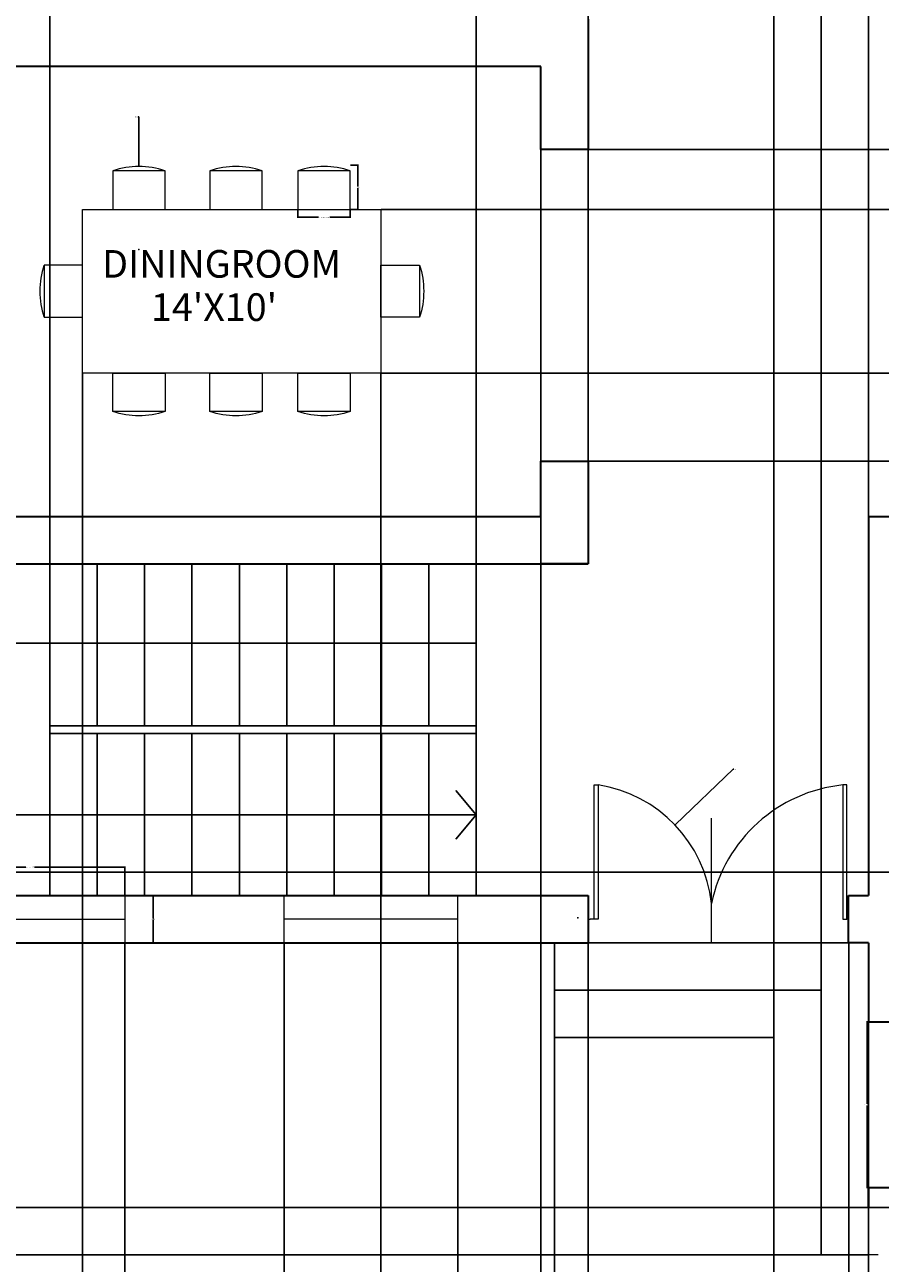
# Model space of a CAD drawing. Units: inches. Extents: x 2863 to 3499, y 1212 to 2136.
# Tile 3 of 7: x 2991 to 3208, y 1372 to 1686. Entities that reach past the tile are written whole.
import ezdxf

# ---------------------------------------------------------------- set-up
doc = ezdxf.new("R2010")
doc.units = ezdxf.units.IN
doc.linetypes.add('DASHED2', pattern=[9.525, 6.35, -3.175])
for name, color, linetype, lineweight in [('A-ANNO-DIMS', 2, 'Continuous', 18), ('A-AREA-IDEN', 7, 'Continuous', 18), ('A-DOOR', 221, 'Continuous', 18), ('A-FLOR-OVHD', 51, 'DASHED2', 18), ('A-FLOR-STRS', 51, 'Continuous', 25), ('A-FURN', 131, 'Continuous', 18), ('A-GLAZ', 191, 'Continuous', 18), ('A-WALL', 51, 'Continuous', 35)]:
    doc.layers.add(name, color=color, linetype=linetype, lineweight=lineweight)
doc.styles.get("Standard").update_dxf_attribs({"font": 'arial.ttf'})
doc.dimstyles.get("Standard").update_dxf_attribs({"dimtxt": 0.18, "dimasz": 0.18, "dimexe": 0.18, "dimexo": 0.0625, "dimgap": 0.09, "dimtad": 0, "dimtih": 1, "dimtoh": 1, "dimdec": 4, "dimzin": 0, "dimdsep": 46, "dimtxsty": 'Standard', "dimcen": 0.09, "dimadec": 0, "dimazin": 0, "dimtfac": 1, "dimtdec": 4, "dimtofl": 0, "dimtmove": 0, "dimatfit": 3, "dimfxl": 1, "dimtolj": 1, "dimtzin": 0, "dimarcsym": 0})

# ---------------------------------------------------------------- blocks, each defined once
blk = doc.blocks.new('CHAIR-DINING')
blk.add_lwpolyline([(0, 0), (13.22, 0), (13.22, 9.77), (0, 9.77)], close=True)
blk.add_arc((6.61, -10.16), 21, 71.6601, 108.3399)
blk = doc.blocks.new('WINDOW-44IN')
for p, q in [((12, 44), (0, 44)), ((6, 44), (6, 0)), ((12, 0), (0, 0))]:
    blk.add_line(p, q)
blk = doc.blocks.new('WINDOW-48IN')
for p, q in [((12, 48), (0, 48)), ((6, 48), (6, 0)), ((12, 0), (0, 0))]:
    blk.add_line(p, q)
blk = doc.blocks.new('*D17')
at = {"layer": 'A-ANNO-DIMS', "color": 0, "lineweight": -2, "transparency": 16777216}
for p, q in [((3060.4, 1638.9), (3060.4, 1636.8)), ((3073.61, 1638.9), (3073.61, 1636.8)), ((3060.58, 1636.98), (3065.58, 1636.98)), ((3073.43, 1636.98), (3068.43, 1636.98))]:
    blk.add_line(p, q, dxfattribs=at)
at = {"layer": 'A-ANNO-DIMS', "color": 0, "transparency": 16777216}
for points in [[(3060.58, 1637.01), (3060.58, 1636.95), (3060.4, 1636.98)], [(3073.43, 1637.01), (3073.43, 1636.95), (3073.61, 1636.98)]]:
    blk.add_solid(points, dxfattribs=at)
at = {"layer": 'Defpoints', "color": 0, "transparency": 16777216}
for p in [(3060.4, 1638.96), (3073.61, 1638.96), (3073.61, 1636.98)]:
    blk.add_point(p, dxfattribs=at)
at = {"layer": 'A-ANNO-DIMS', "color": 0, "transparency": 16777216, "insert": (3067, 1636.98), "char_height": 0.18, "attachment_point": 5}
blk.add_mtext('\\A1;DINING CHAIR 13 TYP.', dxfattribs=at)
blk = doc.blocks.new('*D18')
at = {"layer": 'A-ANNO-DIMS', "color": 0, "lineweight": -2, "transparency": 16777216}
for p, q in [((3073.67, 1650.15), (3075.77, 1650.15)), ((3075.59, 1649.97), (3075.59, 1644.74)), ((3075.59, 1639.14), (3075.59, 1644.37)), ((3073.67, 1638.96), (3075.77, 1638.96))]:
    blk.add_line(p, q, dxfattribs=at)
at = {"layer": 'A-ANNO-DIMS', "color": 0, "transparency": 16777216}
for points in [[(3075.56, 1649.97), (3075.62, 1649.97), (3075.59, 1650.15)], [(3075.56, 1639.14), (3075.62, 1639.14), (3075.59, 1638.96)]]:
    blk.add_solid(points, dxfattribs=at)
at = {"layer": 'Defpoints', "color": 0, "transparency": 16777216}
for p in [(3073.61, 1650.15), (3075.59, 1650.15), (3073.61, 1638.96)]:
    blk.add_point(p, dxfattribs=at)
at = {"layer": 'A-ANNO-DIMS', "color": 0, "transparency": 16777216, "insert": (3075.59, 1644.56), "char_height": 0.18, "attachment_point": 5}
blk.add_mtext('\\A1;11 TYP.', dxfattribs=at)
blk = doc.blocks.new('*D33')
at = {"layer": 'A-ANNO-DIMS', "color": 0, "lineweight": -2, "transparency": 16777216}
for p, q in [((2968.53, 1465.23), (2968.53, 1472.55)), ((2968.71, 1472.37), (2991.41, 1472.37)), ((3016.35, 1472.37), (2993.64, 1472.37)), ((3016.53, 1465.23), (3016.53, 1472.55))]:
    blk.add_line(p, q, dxfattribs=at)
at = {"layer": 'A-ANNO-DIMS', "color": 0, "transparency": 16777216}
for points in [[(2968.71, 1472.4), (2968.71, 1472.34), (2968.53, 1472.37)], [(3016.35, 1472.4), (3016.35, 1472.34), (3016.53, 1472.37)]]:
    blk.add_solid(points, dxfattribs=at)
at = {"layer": 'Defpoints', "color": 0, "transparency": 16777216}
for p in [(2968.53, 1472.37), (2968.53, 1465.17), (3016.53, 1465.17)]:
    blk.add_point(p, dxfattribs=at)
at = {"layer": 'A-ANNO-DIMS', "color": 0, "transparency": 16777216, "insert": (2992.53, 1472.37), "char_height": 0.18, "attachment_point": 5}
blk.add_mtext('\\A1;WINDOW 48 TYP.', dxfattribs=at)
blk = doc.blocks.new('*D34')
at = {"layer": 'A-ANNO-DIMS', "color": 0, "lineweight": -2, "transparency": 16777216}
for p, q in [((3016.59, 1465.17), (3023.91, 1465.17)), ((3023.73, 1464.99), (3023.73, 1459.35)), ((3023.73, 1453.35), (3023.73, 1458.98)), ((3016.59, 1453.17), (3023.91, 1453.17))]:
    blk.add_line(p, q, dxfattribs=at)
at = {"layer": 'A-ANNO-DIMS', "color": 0, "transparency": 16777216}
for points in [[(3023.7, 1464.99), (3023.76, 1464.99), (3023.73, 1465.17)], [(3023.7, 1453.35), (3023.76, 1453.35), (3023.73, 1453.17)]]:
    blk.add_solid(points, dxfattribs=at)
at = {"layer": 'Defpoints', "color": 0, "transparency": 16777216}
for p in [(3016.53, 1465.17), (3023.73, 1465.17), (3016.53, 1453.17)]:
    blk.add_point(p, dxfattribs=at)
at = {"layer": 'A-ANNO-DIMS', "color": 0, "transparency": 16777216, "insert": (3023.73, 1459.17), "char_height": 0.18, "attachment_point": 5}
blk.add_mtext('\\A1;12 TYP.', dxfattribs=at)
blk = doc.blocks.new('*D39')
at = {"layer": 'A-ANNO-DIMS', "color": 0, "lineweight": -2, "transparency": 16777216}
for p, q in [((3210.85, 1433.18), (3204.43, 1433.18)), ((3204.61, 1433), (3204.61, 1412.36)), ((3204.61, 1391.35), (3204.61, 1411.99)), ((3210.85, 1391.17), (3204.43, 1391.17))]:
    blk.add_line(p, q, dxfattribs=at)
at = {"layer": 'A-ANNO-DIMS', "color": 0, "transparency": 16777216}
for points in [[(3204.58, 1433), (3204.64, 1433), (3204.61, 1433.18)], [(3204.58, 1391.35), (3204.64, 1391.35), (3204.61, 1391.17)]]:
    blk.add_solid(points, dxfattribs=at)
at = {"layer": 'Defpoints', "color": 0, "transparency": 16777216}
for p in [(3204.61, 1433.18), (3210.92, 1433.18), (3210.92, 1391.17)]:
    blk.add_point(p, dxfattribs=at)
at = {"layer": 'A-ANNO-DIMS', "color": 0, "transparency": 16777216, "insert": (3204.61, 1412.17), "char_height": 0.18, "attachment_point": 5}
blk.add_mtext('\\A1;DOOR 42 TYP.', dxfattribs=at)
blk = doc.blocks.new('*D69')
at = {"layer": 'A-ANNO-DIMS', "color": 0, "lineweight": -2, "transparency": 16777216}
for p, q in [((3204.85, 1453.17), (2862.72, 1453.17)), ((2862.9, 1452.99), (2862.9, 1413.85)), ((2862.9, 1374.35), (2862.9, 1413.48)), ((3204.85, 1374.17), (2862.72, 1374.17))]:
    blk.add_line(p, q, dxfattribs=at)
at = {"layer": 'A-ANNO-DIMS', "color": 0, "transparency": 16777216}
for points in [[(2862.87, 1452.99), (2862.93, 1452.99), (2862.9, 1453.17)], [(2862.87, 1374.35), (2862.93, 1374.35), (2862.9, 1374.17)]]:
    blk.add_solid(points, dxfattribs=at)
at = {"layer": 'Defpoints', "color": 0, "transparency": 16777216}
for p in [(3204.92, 1453.17), (2862.9, 1374.17), (3204.92, 1374.17)]:
    blk.add_point(p, dxfattribs=at)
at = {"layer": 'A-ANNO-DIMS', "color": 0, "transparency": 16777216, "insert": (2862.9, 1413.67), "char_height": 0.18, "attachment_point": 5}
blk.add_mtext('\\A1;79', dxfattribs=at)
blk = doc.blocks.new('*D70')
at = {"layer": 'A-ANNO-DIMS', "color": 0, "lineweight": -2, "transparency": 16777216}
for p, q in [((2940.92, 1453.1), (2940.92, 1211.97)), ((3204.92, 1374.1), (3204.92, 1211.97)), ((2941.1, 1212.15), (3072.63, 1212.15)), ((3204.74, 1212.15), (3073.21, 1212.15))]:
    blk.add_line(p, q, dxfattribs=at)
at = {"layer": 'A-ANNO-DIMS', "color": 0, "transparency": 16777216}
for points in [[(2941.1, 1212.18), (2941.1, 1212.12), (2940.92, 1212.15)], [(3204.74, 1212.18), (3204.74, 1212.12), (3204.92, 1212.15)]]:
    blk.add_solid(points, dxfattribs=at)
at = {"layer": 'Defpoints', "color": 0, "transparency": 16777216}
for p in [(2940.92, 1453.17), (3204.92, 1374.17), (3204.92, 1212.15)]:
    blk.add_point(p, dxfattribs=at)
at = {"layer": 'A-ANNO-DIMS', "color": 0, "transparency": 16777216, "insert": (3072.92, 1212.15), "char_height": 0.18, "attachment_point": 5}
blk.add_mtext('\\A1;264', dxfattribs=at)
blk = doc.blocks.new('*D71')
at = {"layer": 'A-ANNO-DIMS', "color": 0, "lineweight": -2, "transparency": 16777216}
for p, q in [((3204.92, 1374.1), (3204.92, 1211.97)), ((3420.92, 1374.1), (3420.92, 1211.97)), ((3205.1, 1212.15), (3312.63, 1212.15)), ((3420.74, 1212.15), (3313.21, 1212.15))]:
    blk.add_line(p, q, dxfattribs=at)
at = {"layer": 'A-ANNO-DIMS', "color": 0, "transparency": 16777216}
for points in [[(3205.1, 1212.18), (3205.1, 1212.12), (3204.92, 1212.15)], [(3420.74, 1212.18), (3420.74, 1212.12), (3420.92, 1212.15)]]:
    blk.add_solid(points, dxfattribs=at)
at = {"layer": 'Defpoints', "color": 0, "transparency": 16777216}
for p in [(3204.92, 1374.17), (3420.92, 1374.17), (3420.92, 1212.15)]:
    blk.add_point(p, dxfattribs=at)
at = {"layer": 'A-ANNO-DIMS', "color": 0, "transparency": 16777216, "insert": (3312.92, 1212.15), "char_height": 0.18, "attachment_point": 5}
blk.add_mtext('\\A1;216', dxfattribs=at)
blk = doc.blocks.new('*D72')
at = {"layer": 'A-ANNO-DIMS', "color": 0, "lineweight": -2, "transparency": 16777216}
for p, q in [((3133.92, 1549.23), (3133.92, 2136.37)), ((3204.92, 1561.23), (3204.92, 2136.37)), ((3134.1, 2136.19), (3169.22, 2136.19)), ((3204.74, 2136.19), (3169.62, 2136.19))]:
    blk.add_line(p, q, dxfattribs=at)
at = {"layer": 'A-ANNO-DIMS', "color": 0, "transparency": 16777216}
for points in [[(3134.1, 2136.22), (3134.1, 2136.16), (3133.92, 2136.19)], [(3204.74, 2136.22), (3204.74, 2136.16), (3204.92, 2136.19)]]:
    blk.add_solid(points, dxfattribs=at)
at = {"layer": 'Defpoints', "color": 0, "transparency": 16777216}
for p in [(3204.92, 2136.19), (3204.92, 1561.17), (3133.92, 1549.17)]:
    blk.add_point(p, dxfattribs=at)
at = {"layer": 'A-ANNO-DIMS', "color": 0, "transparency": 16777216, "insert": (3169.42, 2136.19), "char_height": 0.18, "attachment_point": 5}
blk.add_mtext('\\A1;71', dxfattribs=at)
blk = doc.blocks.new('*D74')
at = {"layer": 'A-ANNO-DIMS', "color": 0, "lineweight": -2, "transparency": 16777216}
for p, q in [((3408.85, 1471.09), (2862.72, 1471.09)), ((2862.9, 1470.91), (2862.9, 1428.81)), ((2862.9, 1386.35), (2862.9, 1428.44)), ((3408.85, 1386.17), (2862.72, 1386.17))]:
    blk.add_line(p, q, dxfattribs=at)
at = {"layer": 'A-ANNO-DIMS', "color": 0, "transparency": 16777216}
for points in [[(2862.87, 1470.91), (2862.93, 1470.91), (2862.9, 1471.09)], [(2862.87, 1386.35), (2862.93, 1386.35), (2862.9, 1386.17)]]:
    blk.add_solid(points, dxfattribs=at)
at = {"layer": 'Defpoints', "color": 0, "transparency": 16777216}
for p in [(3408.92, 1471.09), (2862.9, 1386.17), (3408.92, 1386.17)]:
    blk.add_point(p, dxfattribs=at)
at = {"layer": 'A-ANNO-DIMS', "color": 0, "transparency": 16777216, "insert": (2862.9, 1428.63), "char_height": 0.18, "attachment_point": 5}
blk.add_mtext('\\A1;84.92', dxfattribs=at)
blk = doc.blocks.new('*D76')
at = {"layer": 'A-ANNO-DIMS', "color": 0, "lineweight": -2, "transparency": 16777216}
for p, q in [((2952.92, 1675.1), (2952.92, 1211.97)), ((3121.92, 1675.1), (3121.92, 1211.97)), ((2953.1, 1212.15), (3037.14, 1212.15)), ((3121.74, 1212.15), (3037.7, 1212.15))]:
    blk.add_line(p, q, dxfattribs=at)
at = {"layer": 'A-ANNO-DIMS', "color": 0, "transparency": 16777216}
for points in [[(2953.1, 1212.18), (2953.1, 1212.12), (2952.92, 1212.15)], [(3121.74, 1212.18), (3121.74, 1212.12), (3121.92, 1212.15)]]:
    blk.add_solid(points, dxfattribs=at)
at = {"layer": 'Defpoints', "color": 0, "transparency": 16777216}
for p in [(2952.92, 1675.17), (3121.92, 1675.17), (3121.92, 1212.15)]:
    blk.add_point(p, dxfattribs=at)
at = {"layer": 'A-ANNO-DIMS', "color": 0, "transparency": 16777216, "insert": (3037.42, 1212.15), "char_height": 0.18, "attachment_point": 5}
blk.add_mtext('\\A1;169', dxfattribs=at)
blk = doc.blocks.new('*D77')
at = {"layer": 'A-ANNO-DIMS', "color": 0, "lineweight": -2, "transparency": 16777216}
for p, q in [((2997.55, 1549.23), (2997.55, 2136.37)), ((3105.55, 1549.23), (3105.55, 2136.37)), ((2997.73, 2136.19), (3051.27, 2136.19)), ((3105.37, 2136.19), (3051.83, 2136.19))]:
    blk.add_line(p, q, dxfattribs=at)
at = {"layer": 'A-ANNO-DIMS', "color": 0, "transparency": 16777216}
for points in [[(2997.73, 2136.22), (2997.73, 2136.16), (2997.55, 2136.19)], [(3105.37, 2136.22), (3105.37, 2136.16), (3105.55, 2136.19)]]:
    blk.add_solid(points, dxfattribs=at)
at = {"layer": 'Defpoints', "color": 0, "transparency": 16777216}
for p in [(3105.55, 2136.19), (2997.55, 1549.17), (3105.55, 1549.17)]:
    blk.add_point(p, dxfattribs=at)
at = {"layer": 'A-ANNO-DIMS', "color": 0, "transparency": 16777216, "insert": (3051.55, 2136.19), "char_height": 0.18, "attachment_point": 5}
blk.add_mtext('\\A1;108', dxfattribs=at)
blk = doc.blocks.new('*D79')
at = {"layer": 'A-ANNO-DIMS', "color": 0, "lineweight": -2, "transparency": 16777216}
for p, q in [((3005.82, 1597.44), (3005.82, 1211.97)), ((3081.41, 1597.44), (3081.41, 1211.97)), ((3006, 1212.15), (3043.23, 1212.15)), ((3081.23, 1212.15), (3044.01, 1212.15))]:
    blk.add_line(p, q, dxfattribs=at)
at = {"layer": 'A-ANNO-DIMS', "color": 0, "transparency": 16777216}
for points in [[(3006, 1212.18), (3006, 1212.12), (3005.82, 1212.15)], [(3081.23, 1212.18), (3081.23, 1212.12), (3081.41, 1212.15)]]:
    blk.add_solid(points, dxfattribs=at)
at = {"layer": 'Defpoints', "color": 0, "transparency": 16777216}
for p in [(3005.82, 1597.5), (3081.41, 1597.5), (3081.41, 1212.15)]:
    blk.add_point(p, dxfattribs=at)
at = {"layer": 'A-ANNO-DIMS', "color": 0, "transparency": 16777216, "insert": (3043.62, 1212.15), "char_height": 0.18, "attachment_point": 5}
blk.add_mtext('\\A1;75.59', dxfattribs=at)
blk = doc.blocks.new('*D80')
at = {"layer": 'A-ANNO-DIMS', "color": 0, "lineweight": -2, "transparency": 16777216}
for p, q in [((3081.48, 1638.96), (3499.12, 1638.96)), ((3498.94, 1638.78), (3498.94, 1618.41)), ((3498.94, 1597.68), (3498.94, 1618.05)), ((3081.48, 1597.5), (3499.12, 1597.5))]:
    blk.add_line(p, q, dxfattribs=at)
at = {"layer": 'A-ANNO-DIMS', "color": 0, "transparency": 16777216}
for points in [[(3498.91, 1638.78), (3498.97, 1638.78), (3498.94, 1638.96)], [(3498.91, 1597.68), (3498.97, 1597.68), (3498.94, 1597.5)]]:
    blk.add_solid(points, dxfattribs=at)
at = {"layer": 'Defpoints', "color": 0, "transparency": 16777216}
for p in [(3081.41, 1638.96), (3498.94, 1638.96), (3081.41, 1597.5)]:
    blk.add_point(p, dxfattribs=at)
at = {"layer": 'A-ANNO-DIMS', "color": 0, "transparency": 16777216, "insert": (3498.94, 1618.23), "char_height": 0.18, "attachment_point": 5}
blk.add_mtext('\\A1;41.46', dxfattribs=at)
blk = doc.blocks.new('*D81')
at = {"layer": 'A-ANNO-DIMS', "color": 0, "lineweight": -2, "transparency": 16777216}
for p, q in [((3133.92, 1453.1), (3133.92, 1211.97)), ((3199.92, 1453.1), (3199.92, 1211.97)), ((3134.1, 1212.15), (3166.7, 1212.15)), ((3199.74, 1212.15), (3167.14, 1212.15))]:
    blk.add_line(p, q, dxfattribs=at)
at = {"layer": 'A-ANNO-DIMS', "color": 0, "transparency": 16777216}
for points in [[(3134.1, 1212.18), (3134.1, 1212.12), (3133.92, 1212.15)], [(3199.74, 1212.18), (3199.74, 1212.12), (3199.92, 1212.15)]]:
    blk.add_solid(points, dxfattribs=at)
at = {"layer": 'Defpoints', "color": 0, "transparency": 16777216}
for p in [(3133.92, 1453.17), (3199.92, 1453.17), (3199.92, 1212.15)]:
    blk.add_point(p, dxfattribs=at)
at = {"layer": 'A-ANNO-DIMS', "color": 0, "transparency": 16777216, "insert": (3166.92, 1212.15), "char_height": 0.18, "attachment_point": 5}
blk.add_mtext('\\A1;66', dxfattribs=at)
blk = doc.blocks.new('*D82')
at = {"layer": 'A-ANNO-DIMS', "color": 0, "lineweight": -2, "transparency": 16777216}
for p, q in [((3121.98, 1654.17), (3499.12, 1654.17)), ((3498.94, 1653.99), (3498.94, 1614.85)), ((3498.94, 1575.35), (3498.94, 1614.48)), ((3121.98, 1575.17), (3499.12, 1575.17))]:
    blk.add_line(p, q, dxfattribs=at)
at = {"layer": 'A-ANNO-DIMS', "color": 0, "transparency": 16777216}
for points in [[(3498.91, 1653.99), (3498.97, 1653.99), (3498.94, 1654.17)], [(3498.91, 1575.35), (3498.97, 1575.35), (3498.94, 1575.17)]]:
    blk.add_solid(points, dxfattribs=at)
at = {"layer": 'Defpoints', "color": 0, "transparency": 16777216}
for p in [(3121.92, 1654.17), (3498.94, 1654.17), (3121.92, 1575.17)]:
    blk.add_point(p, dxfattribs=at)
at = {"layer": 'A-ANNO-DIMS', "color": 0, "transparency": 16777216, "insert": (3498.94, 1614.67), "char_height": 0.18, "attachment_point": 5}
blk.add_mtext('\\A1;79', dxfattribs=at)
blk = doc.blocks.new('*D102')
at = {"layer": 'A-ANNO-DIMS', "color": 0, "lineweight": -2, "transparency": 16777216}
for p, q in [((3016.53, 1453.1), (3016.53, 1211.97)), ((3056.9, 1453.1), (3056.9, 1211.97)), ((3016.71, 1212.15), (3036.31, 1212.15)), ((3056.72, 1212.15), (3037.11, 1212.15))]:
    blk.add_line(p, q, dxfattribs=at)
at = {"layer": 'A-ANNO-DIMS', "color": 0, "transparency": 16777216}
for points in [[(3016.71, 1212.18), (3016.71, 1212.12), (3016.53, 1212.15)], [(3056.72, 1212.18), (3056.72, 1212.12), (3056.9, 1212.15)]]:
    blk.add_solid(points, dxfattribs=at)
at = {"layer": 'Defpoints', "color": 0, "transparency": 16777216}
for p in [(3016.53, 1453.17), (3056.9, 1453.17), (3056.9, 1212.15)]:
    blk.add_point(p, dxfattribs=at)
at = {"layer": 'A-ANNO-DIMS', "color": 0, "transparency": 16777216, "insert": (3036.71, 1212.15), "char_height": 0.18, "attachment_point": 5}
blk.add_mtext('\\A1;40.37', dxfattribs=at)
blk = doc.blocks.new('*D103')
at = {"layer": 'A-ANNO-DIMS', "color": 0, "lineweight": -2, "transparency": 16777216}
for p, q in [((3100.9, 1453.1), (3100.9, 1211.97)), ((3133.92, 1453.1), (3133.92, 1211.97)), ((3101.08, 1212.15), (3117.01, 1212.15)), ((3133.74, 1212.15), (3117.8, 1212.15))]:
    blk.add_line(p, q, dxfattribs=at)
at = {"layer": 'A-ANNO-DIMS', "color": 0, "transparency": 16777216}
for points in [[(3101.08, 1212.18), (3101.08, 1212.12), (3100.9, 1212.15)], [(3133.74, 1212.18), (3133.74, 1212.12), (3133.92, 1212.15)]]:
    blk.add_solid(points, dxfattribs=at)
at = {"layer": 'Defpoints', "color": 0, "transparency": 16777216}
for p in [(3100.9, 1453.17), (3133.92, 1453.17), (3133.92, 1212.15)]:
    blk.add_point(p, dxfattribs=at)
at = {"layer": 'A-ANNO-DIMS', "color": 0, "transparency": 16777216, "insert": (3117.41, 1212.15), "char_height": 0.18, "attachment_point": 5}
blk.add_mtext('\\A1;33.02', dxfattribs=at)
blk = doc.blocks.new('*D109')
at = {"layer": 'A-ANNO-DIMS', "color": 0, "lineweight": -2, "transparency": 16777216}
for p, q in [((3125.36, 1429.1), (3125.36, 1211.97)), ((3180.92, 1429.1), (3180.92, 1211.97)), ((3125.54, 1212.15), (3152.74, 1212.15)), ((3180.74, 1212.15), (3153.53, 1212.15))]:
    blk.add_line(p, q, dxfattribs=at)
at = {"layer": 'A-ANNO-DIMS', "color": 0, "transparency": 16777216}
for points in [[(3125.54, 1212.18), (3125.54, 1212.12), (3125.36, 1212.15)], [(3180.74, 1212.18), (3180.74, 1212.12), (3180.92, 1212.15)]]:
    blk.add_solid(points, dxfattribs=at)
at = {"layer": 'Defpoints', "color": 0, "transparency": 16777216}
for p in [(3125.36, 1429.17), (3180.92, 1429.17), (3180.92, 1212.15)]:
    blk.add_point(p, dxfattribs=at)
at = {"layer": 'A-ANNO-DIMS', "color": 0, "transparency": 16777216, "insert": (3153.14, 1212.15), "char_height": 0.18, "attachment_point": 5}
blk.add_mtext('\\A1;55.56', dxfattribs=at)
blk = doc.blocks.new('*D110')
at = {"layer": 'A-ANNO-DIMS', "color": 0, "lineweight": -2, "transparency": 16777216}
for p, q in [((3180.92, 1374.23), (3180.92, 2136.37)), ((3192.92, 1374.23), (3192.92, 2136.37)), ((3181.1, 2136.19), (3186.71, 2136.19)), ((3192.74, 2136.19), (3187.13, 2136.19))]:
    blk.add_line(p, q, dxfattribs=at)
at = {"layer": 'A-ANNO-DIMS', "color": 0, "transparency": 16777216}
for points in [[(3181.1, 2136.22), (3181.1, 2136.16), (3180.92, 2136.19)], [(3192.74, 2136.22), (3192.74, 2136.16), (3192.92, 2136.19)]]:
    blk.add_solid(points, dxfattribs=at)
at = {"layer": 'Defpoints', "color": 0, "transparency": 16777216}
for p in [(3192.92, 2136.19), (3180.92, 1374.17), (3192.92, 1374.17)]:
    blk.add_point(p, dxfattribs=at)
at = {"layer": 'A-ANNO-DIMS', "color": 0, "transparency": 16777216, "insert": (3186.92, 2136.19), "char_height": 0.18, "attachment_point": 5}
blk.add_mtext('\\A1;12', dxfattribs=at)
blk = doc.blocks.new('*D111')
at = {"layer": 'A-ANNO-DIMS', "color": 0, "lineweight": -2, "transparency": 16777216}
for p, q in [((2952.92, 1549.23), (2952.92, 2136.37)), ((2997.55, 1549.23), (2997.55, 2136.37)), ((2953.1, 2136.19), (2974.83, 2136.19)), ((2997.37, 2136.19), (2975.63, 2136.19))]:
    blk.add_line(p, q, dxfattribs=at)
at = {"layer": 'A-ANNO-DIMS', "color": 0, "transparency": 16777216}
for points in [[(2953.1, 2136.22), (2953.1, 2136.16), (2952.92, 2136.19)], [(2997.37, 2136.22), (2997.37, 2136.16), (2997.55, 2136.19)]]:
    blk.add_solid(points, dxfattribs=at)
at = {"layer": 'Defpoints', "color": 0, "transparency": 16777216}
for p in [(2997.55, 2136.19), (2952.92, 1549.17), (2997.55, 1549.17)]:
    blk.add_point(p, dxfattribs=at)
at = {"layer": 'A-ANNO-DIMS', "color": 0, "transparency": 16777216, "insert": (2975.23, 2136.19), "char_height": 0.18, "attachment_point": 5}
blk.add_mtext('\\A1;44.63', dxfattribs=at)
blk = doc.blocks.new('*D115')
at = {"layer": 'A-ANNO-DIMS', "color": 0, "lineweight": -2, "transparency": 16777216}
for p, q in [((3170.64, 1497.15), (3156.03, 1483.17)), ((3170.82, 1497.15), (3170.64, 1497.15)), ((3131.24, 1459.55), (3131.42, 1459.55)), ((3131.33, 1459.46), (3131.33, 1459.64))]:
    blk.add_line(p, q, dxfattribs=at)
at = {"layer": 'A-ANNO-DIMS', "color": 0, "transparency": 16777216}
blk.add_solid([(3156.01, 1483.2), (3156.05, 1483.15), (3155.9, 1483.05)], dxfattribs=at)
at = {"layer": 'Defpoints', "color": 0, "transparency": 16777216}
for p in [(3155.9, 1483.05), (3131.33, 1459.55)]:
    blk.add_point(p, dxfattribs=at)
at = {"layer": 'A-ANNO-DIMS', "color": 0, "transparency": 16777216, "insert": (3171.12, 1497.15), "char_height": 0.18, "attachment_point": 5}
blk.add_mtext('\\A1;R34', dxfattribs=at)
blk = doc.blocks.new('*D119')
at = {"layer": 'A-ANNO-DIMS', "color": 0, "lineweight": -2, "transparency": 16777216}
for p, q in [((3019.91, 1662.4), (3020.09, 1662.4)), ((3020.09, 1662.4), (3020.09, 1649.98)), ((3020.01, 1628.8), (3020.19, 1628.8)), ((3020.1, 1628.71), (3020.1, 1628.89))]:
    blk.add_line(p, q, dxfattribs=at)
at = {"layer": 'A-ANNO-DIMS', "color": 0, "transparency": 16777216}
blk.add_solid([(3020.12, 1649.98), (3020.06, 1649.98), (3020.09, 1649.8)], dxfattribs=at)
at = {"layer": 'Defpoints', "color": 0, "transparency": 16777216}
for p in [(3020.09, 1649.8), (3020.1, 1628.8)]:
    blk.add_point(p, dxfattribs=at)
at = {"layer": 'A-ANNO-DIMS', "color": 0, "transparency": 16777216, "insert": (3019.43, 1662.4), "char_height": 0.18, "attachment_point": 5}
blk.add_mtext('\\A1;4X R21', dxfattribs=at)

msp = doc.modelspace()

# ---------------------------------------------------------------- linework, layer by layer
at = {"layer": 'A-DOOR'}
for p, q in [((3135.4168, 1459.1651), (3135.4168, 1493.1651)), ((3135.4168, 1493.1651), (3136.4168, 1493.1651)), ((3136.4168, 1493.1651), (3136.4168, 1459.1651)), ((3199.4168, 1493.1651), (3198.4168, 1493.1651)), ((3198.4168, 1493.1651), (3198.4168, 1459.1651)), ((3199.4168, 1459.1651), (3199.4168, 1493.1651)), ((3165.1366, 1453.1651), (3165.1366, 1484.7256)), ((3133.9168, 1459.1651), (3134.4168, 1459.1651)), ((3135.4168, 1459.1651), (3134.4168, 1459.1651)), ((3136.4168, 1459.1651), (3135.4168, 1459.1651)), ((3198.4168, 1459.1651), (3199.4168, 1459.1651)), ((3199.9168, 1459.1651), (3199.4168, 1459.1651))]:
    msp.add_line(p, q, dxfattribs=at)
for centre, radius, start, end in [((3131.3266, 1459.5483), 34, 6.059429, 81.389827), ((3202.3338, 1455.3675), 38, 95.916573, 168.201616)]:
    msp.add_arc(centre, radius, start, end, dxfattribs=at)
at = {"layer": 'A-FLOR-OVHD'}
for p, q in [((3121.9168, 1654.1651), (3121.9168, 1575.1651)), ((3133.9168, 1654.1651), (3133.9168, 1575.1651)), ((2952.9168, 1386.1651), (3204.9168, 1386.1651)), ((3216.9168, 1374.1651), (2940.9168, 1374.1651))]:
    msp.add_line(p, q, dxfattribs=at)
at = {"layer": 'A-FLOR-STRS'}
for p, q in [((2997.5458, 1549.1651), (2997.5458, 1465.1651)), ((3009.5458, 1549.1651), (3009.5458, 1508.1651)), ((3021.5458, 1549.1651), (3021.5458, 1508.1651)), ((3033.5458, 1549.1651), (3033.5458, 1508.1651)), ((3045.5458, 1549.1651), (3045.5458, 1508.1651)), ((3057.5458, 1549.1651), (3057.5458, 1508.1651)), ((3069.5458, 1549.1651), (3069.5458, 1508.1651)), ((3081.5458, 1549.1651), (3081.5458, 1508.1651)), ((3093.5458, 1549.1651), (3093.5458, 1508.1651)), ((3105.5458, 1549.1651), (3105.5458, 1465.1651)), ((3105.5458, 1529.0656), (2976.4727, 1529.0656)), ((3105.5458, 1508.1651), (2997.5458, 1508.1651)), ((3105.5458, 1506.1651), (2997.5458, 1506.1651)), ((3009.5458, 1506.1651), (3009.5458, 1465.1651)), ((3021.5458, 1506.1651), (3021.5458, 1465.1651)), ((3033.5458, 1506.1651), (3033.5458, 1465.1651)), ((3045.5458, 1506.1651), (3045.5458, 1465.1651)), ((3057.5458, 1506.1651), (3057.5458, 1465.1651)), ((3069.5458, 1506.1651), (3069.5458, 1465.1651)), ((3081.5458, 1506.1651), (3081.5458, 1465.1651)), ((3093.5458, 1506.1651), (3093.5458, 1465.1651)), ((3105.5458, 1485.602), (3100.4035, 1491.7303)), ((2976.4727, 1485.602), (3105.5458, 1485.602)), ((3105.5458, 1485.602), (3100.4035, 1479.4736)), ((3125.3565, 1453.1651), (3204.9168, 1453.1651)), ((3125.3565, 1441.1651), (3125.3565, 1453.1651)), ((3204.9168, 1453.1651), (3204.9168, 1374.1651)), ((3192.9168, 1441.1651), (3125.3565, 1441.1651)), ((3125.3565, 1429.1651), (3125.3565, 1441.1651)), ((3192.9168, 1374.1651), (3192.9168, 1441.1651)), ((3180.9168, 1429.1651), (3125.3565, 1429.1651)), ((3180.9168, 1374.1651), (3180.9168, 1429.1651)), ((3192.9168, 1374.1651), (3180.9168, 1374.1651)), ((3204.9168, 1374.1651), (3192.9168, 1374.1651))]:
    msp.add_line(p, q, dxfattribs=at)
at = {"layer": 'A-FURN'}
msp.add_lwpolyline([(3005.8227, 1638.9588), (3081.415, 1638.9588), (3081.415, 1597.4979), (3005.8227, 1597.4979)], close=True, dxfattribs=at)
at = {"layer": 'A-WALL'}
for p, q in [((3133.9168, 1687.1651), (3133.9168, 1675.1651)), ((3121.9168, 1675.1651), (2952.9168, 1675.1651)), ((3121.9168, 1654.1651), (3121.9168, 1675.1651)), ((3133.9168, 1675.1651), (3133.9168, 1654.1651)), ((3133.9168, 1654.1651), (3121.9168, 1654.1651)), ((3121.9168, 1561.1651), (3121.9168, 1575.1651)), ((3121.9168, 1575.1651), (3133.9168, 1575.1651)), ((3133.9168, 1575.1651), (3133.9168, 1549.1651)), ((2952.9168, 1561.1651), (3121.9168, 1561.1651)), ((3204.9168, 1561.1651), (3204.9168, 1465.1651)), ((3204.9168, 1561.1651), (3219.9168, 1561.1651)), ((3204.9168, 1561.1651), (3219.9168, 1561.1651)), ((2952.9168, 1549.1651), (3133.9168, 1549.1651)), ((3133.9168, 1549.1651), (3121.9168, 1549.1651)), ((2952.9168, 1465.1651), (3133.9168, 1465.1651)), ((3133.9168, 1465.1651), (3133.9168, 1453.1651)), ((3199.9168, 1453.1651), (3199.9168, 1465.1651)), ((3199.9168, 1465.1651), (3204.9168, 1465.1651)), ((2940.9168, 1453.1651), (3133.9168, 1453.1651)), ((3204.9168, 1453.1651), (3199.9168, 1453.1651)), ((3204.9168, 1453.1651), (3204.9168, 1446.4907)), ((3204.9168, 1453.1651), (3204.9168, 1433.1651)), ((3204.9168, 1433.1651), (3216.9168, 1433.1651)), ((3204.9168, 1386.1651), (3204.9168, 1391.1651)), ((3204.9168, 1391.1651), (3216.9168, 1391.1651)), ((3204.9168, 1391.1651), (3204.9168, 1386.1651))]:
    msp.add_line(p, q, dxfattribs=at)

# ---------------------------------------------------------------- block references
at = {"layer": 'A-FURN'}
for p in [(3013.488, 1638.959), (3038.0687, 1638.959), (3060.3974, 1638.959)]:
    msp.add_blockref('CHAIR-DINING', p, dxfattribs=at)
at = {"layer": 'A-FURN', "rotation": 90.00000000000101}
msp.add_blockref('CHAIR-DINING', (3005.8224, 1611.621), dxfattribs=at)
at = {"layer": 'A-FURN', "extrusion": (0, 0, -1), "zscale": -1}
for p, rotation in [((-3081.4152, 1611.621), 90.00000000000101), ((-3013.488, 1597.4977), 180), ((-3038.0687, 1597.4977), 180), ((-3060.3974, 1597.4977), 180)]:
    msp.add_blockref('CHAIR-DINING', p, dxfattribs=dict(at, rotation=rotation))
at = {"layer": 'A-GLAZ'}
for name, p, rotation in [('WINDOW-48IN', (3016.5255, 1453.1653), 89.9999999999968), ('WINDOW-44IN', (3056.8975, 1465.1648), 269.9999999999993)]:
    msp.add_blockref(name, p, dxfattribs=dict(at, rotation=rotation))

# ---------------------------------------------------------------- texts
at = {"layer": 'A-AREA-IDEN'}
for tag, p in [('DININGROOM', (3010.7843, 1621.6608)), ("14'X10'", (3023.1386, 1610.7015))]:
    msp.add_attdef(tag, p, '', height=7, dxfattribs=at)

# ---------------------------------------------------------------- dimensions: what is measured, and where the dimension line sits
at = {"layer": 'A-ANNO-DIMS'}
for base, p1, p2, override, picture, middle in [((2997.5458, 2136.1851), (2952.9168, 1549.1651), (2997.5458, 1549.1651), {"dimdec": 2, "dimlfac": 1, "dimrnd": 0, "dimzin": 0, "dimdsep": 46, "dimlunit": 2}, '*D111', (2975.2313, 2136.1851)), ((3105.5458, 2136.1851), (2997.5458, 1549.1651), (3105.5458, 1549.1651), {"dimdec": 0, "dimlfac": 1, "dimrnd": 0, "dimzin": 0, "dimdsep": 46, "dimlunit": 2}, '*D77', (3051.5458, 2136.1851)), ((3204.9168, 2136.1851), (3133.9168, 1549.1651), (3204.9168, 1561.1651), {"dimdec": 0, "dimlfac": 1, "dimrnd": 0, "dimzin": 0, "dimdsep": 46, "dimlunit": 2}, '*D72', (3169.4168, 2136.1851)), ((3192.9168, 2136.1851), (3180.9168, 1374.1651), (3192.9168, 1374.1651), {"dimdec": 0, "dimlfac": 1, "dimrnd": 0, "dimzin": 0, "dimdsep": 46, "dimlunit": 2}, '*D110', (3186.9168, 2136.1851)), ((3121.9168, 1212.1451), (2952.9168, 1675.1651), (3121.9168, 1675.1651), {"dimdec": 0, "dimlfac": 1, "dimrnd": 0, "dimzin": 0, "dimdsep": 46, "dimlunit": 2}, '*D76', (3037.4168, 1212.1451)), ((3081.415, 1212.1451), (3005.8227, 1597.4979), (3081.415, 1597.4979), {"dimdec": 2, "dimlfac": 1, "dimrnd": 0, "dimzin": 0, "dimdsep": 46, "dimlunit": 2}, '*D79', (3043.6188, 1212.1451)), ((3204.9168, 1212.1451), (2940.9168, 1453.1651), (3204.9168, 1374.1651), {"dimdec": 0, "dimlfac": 1, "dimrnd": 0, "dimzin": 0, "dimdsep": 46, "dimlunit": 2}, '*D70', (3072.9168, 1212.1451)), ((3056.8973, 1212.1451), (3016.5255, 1453.1651), (3056.8973, 1453.1651), {"dimdec": 2, "dimlfac": 1, "dimrnd": 0, "dimzin": 0, "dimdsep": 46, "dimlunit": 2}, '*D102', (3036.7114, 1212.1451)), ((3133.9168, 1212.1451), (3100.8973, 1453.1651), (3133.9168, 1453.1651), {"dimdec": 2, "dimlfac": 1, "dimrnd": 0, "dimzin": 0, "dimdsep": 46, "dimlunit": 2}, '*D103', (3117.407, 1212.1451)), ((3199.9168, 1212.1451), (3133.9168, 1453.1651), (3199.9168, 1453.1651), {"dimdec": 0, "dimlfac": 1, "dimrnd": 0, "dimzin": 0, "dimdsep": 46, "dimlunit": 2}, '*D81', (3166.9168, 1212.1451)), ((3180.9168, 1212.1451), (3125.3565, 1429.1651), (3180.9168, 1429.1651), {"dimdec": 2, "dimlfac": 1, "dimrnd": 0, "dimzin": 0, "dimdsep": 46, "dimlunit": 2}, '*D109', (3153.1366, 1212.1451)), ((3420.9168, 1212.1451), (3204.9168, 1374.1651), (3420.9168, 1374.1651), {"dimdec": 0, "dimlfac": 1, "dimrnd": 0, "dimzin": 0, "dimdsep": 46, "dimlunit": 2}, '*D71', (3312.9168, 1212.1451))]:
    dim = msp.add_linear_dim(base=base, p1=p1, p2=p2, dimstyle='Standard', override=override, dxfattribs=at)
    dim.commit()
    dim.dimension.update_dxf_attribs({"geometry": picture, "text_midpoint": middle})
dim = msp.add_radius_dim(center=(3020.0953, 1628.7964), mpoint=(3020.095, 1649.7964), text='4X <>', dimstyle='Standard', override={"dimdec": 0, "dimlfac": 1, "dimrnd": 0, "dimzin": 0, "dimdsep": 46, "dimlunit": 2}, dxfattribs=at)
dim.commit()
dim.dimension.update_dxf_attribs({"geometry": '*D119', "text_midpoint": (3019.4301, 1662.3964), "dimtype": 164})
for base, p1, p2, override, picture, middle in [((3498.9368, 1654.1651), (3121.9168, 1575.1651), (3121.9168, 1654.1651), {"dimdec": 0, "dimlfac": 1, "dimrnd": 0, "dimzin": 0, "dimdsep": 46, "dimlunit": 2}, '*D82', (3498.9368, 1614.6651)), ((3498.9368, 1638.9588), (3081.415, 1597.4979), (3081.415, 1638.9588), {"dimdec": 2, "dimlfac": 1, "dimrnd": 0, "dimzin": 0, "dimdsep": 46, "dimlunit": 2}, '*D80', (3498.9368, 1618.2284)), ((2862.8968, 1386.1651), (3408.9168, 1471.0882), (3408.9168, 1386.1651), {"dimdec": 2, "dimlfac": 1, "dimrnd": 0, "dimzin": 0, "dimdsep": 46, "dimlunit": 2}, '*D74', (2862.8968, 1428.6266)), ((2862.8968, 1374.1651), (3204.9168, 1453.1651), (3204.9168, 1374.1651), {"dimdec": 0, "dimlfac": 1, "dimrnd": 0, "dimzin": 0, "dimdsep": 46, "dimlunit": 2}, '*D69', (2862.8968, 1413.6651))]:
    dim = msp.add_linear_dim(base=base, p1=p1, p2=p2, angle=90, dimstyle='Standard', override=override, dxfattribs=at)
    dim.commit()
    dim.dimension.update_dxf_attribs({"geometry": picture, "text_midpoint": middle})
for base, p1, p2, angle, text, picture, middle in [((3075.5948, 1650.152), (3073.6125, 1638.9588), (3073.6125, 1650.152), 90, '<> TYP.', '*D18', (3075.5948, 1644.5554)), ((2968.5255, 1472.3651), (3016.5255, 1465.1651), (2968.5255, 1465.1651), 180, 'WINDOW <> TYP.', '*D33', (2992.5255, 1472.3651)), ((3023.7255, 1465.1651), (3016.5255, 1453.1651), (3016.5255, 1465.1651), 90, '<> TYP.', '*D34', (3023.7255, 1459.1651)), ((3204.6146, 1433.1795), (3210.9168, 1391.1651), (3210.9168, 1433.1795), 90, 'DOOR <> TYP.', '*D39', (3204.6146, 1412.1723))]:
    dim = msp.add_linear_dim(base=base, p1=p1, p2=p2, angle=angle, text=text, dimstyle='Standard', override={"dimdec": 0, "dimlfac": 1, "dimrnd": 0, "dimzin": 0, "dimdsep": 46, "dimlunit": 2}, dxfattribs=at)
    dim.commit()
    dim.dimension.update_dxf_attribs({"geometry": picture, "text_midpoint": middle})
dim = msp.add_linear_dim(base=(3073.6125, 1636.9764), p1=(3060.397, 1638.9588), p2=(3073.6125, 1638.9588), text='DINING CHAIR <> TYP.', dimstyle='Standard', override={"dimdec": 0, "dimlfac": 1, "dimrnd": 0, "dimzin": 0, "dimdsep": 46, "dimlunit": 2}, dxfattribs=at)
dim.commit()
dim.dimension.update_dxf_attribs({"geometry": '*D17', "text_midpoint": (3067.0047, 1636.9764)})
dim = msp.add_radius_dim(center=(3131.3266, 1459.5483), mpoint=(3155.8971, 1483.0491), dimstyle='Standard', override={"dimdec": 0, "dimlfac": 1, "dimrnd": 0, "dimzin": 0, "dimdsep": 46, "dimlunit": 2}, dxfattribs=at)
dim.commit()
dim.dimension.update_dxf_attribs({"geometry": '*D115', "text_midpoint": (3171.1241, 1497.1496), "dimtype": 164})

doc.saveas('drawing.dxf')
